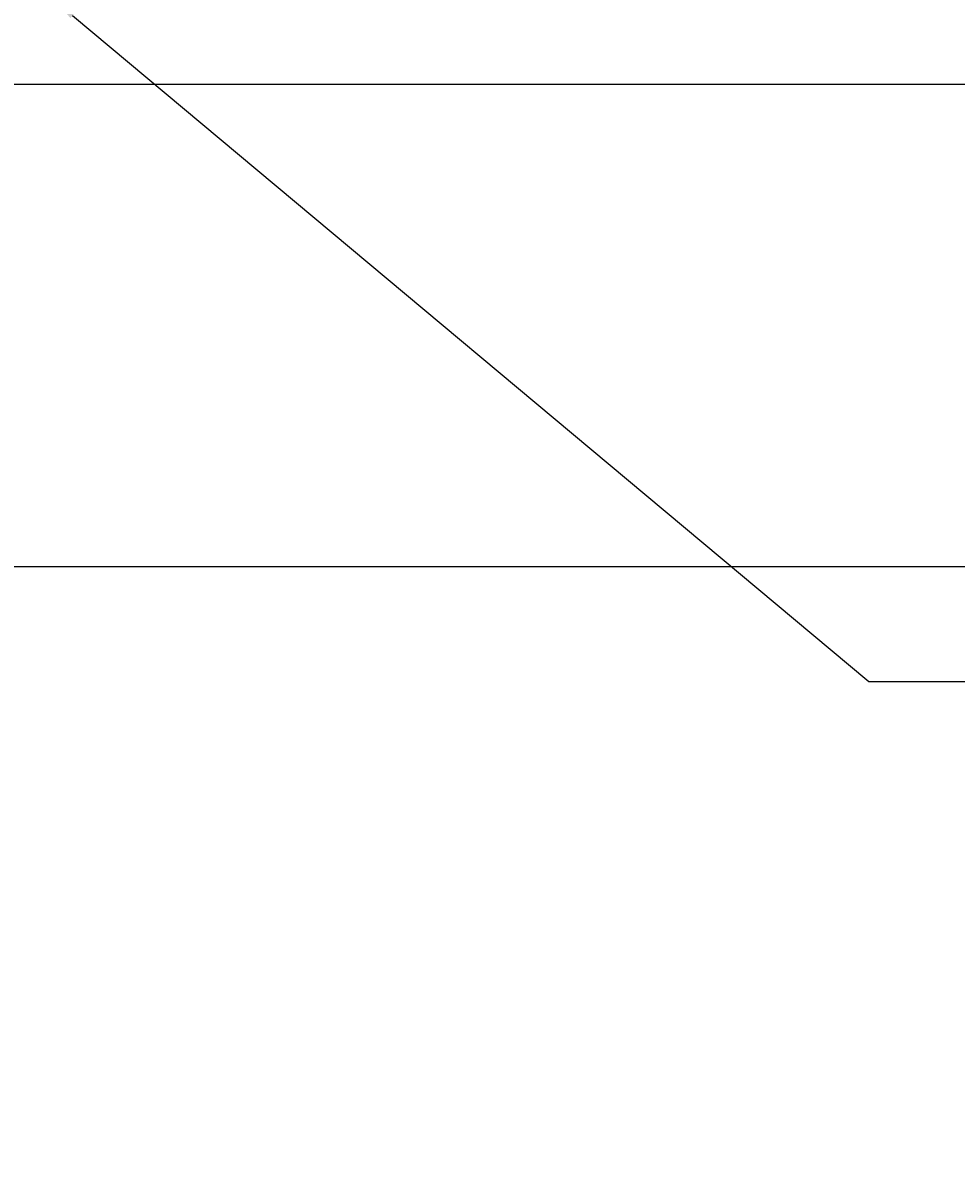
# Model space of a CAD drawing. Units: inches. Extents: x -12 to 334, y -10 to 186.
# Tile 9 of 77: x 42 to 74, y -6 to 33. Entities that reach past the tile are written whole.
import ezdxf
from ezdxf import colors
from ezdxf.entities.mleader import LeaderData, LeaderLine
from ezdxf.math import Vec2, Vec3

# ---------------------------------------------------------------- set-up
doc = ezdxf.new("R2010")
doc.units = ezdxf.units.IN
doc.header["$MEASUREMENT"] = 0
doc.layers.add('M-ANNO-TEXT', color=3, linetype='Continuous', lineweight=25)
doc.layers.add('M-DIMS', color=2, linetype='Continuous', lineweight=18)
doc.styles.get("Standard").update_dxf_attribs({"font": 'arial.ttf'})
doc.dimstyles.get("Standard").update_dxf_attribs({"dimtxt": 0.18, "dimasz": 0.18, "dimexe": 0.18, "dimexo": 0.0625, "dimgap": 0.09, "dimtad": 0, "dimtih": 1, "dimtoh": 1, "dimdec": 4, "dimzin": 0, "dimdsep": 46, "dimtxsty": 'Standard', "dimcen": 0.09, "dimadec": 0, "dimazin": 0, "dimtfac": 1, "dimtdec": 4, "dimtofl": 0, "dimtmove": 0, "dimatfit": 3, "dimfxl": 1, "dimtolj": 1, "dimtzin": 0, "dimarcsym": 0})

# ---------------------------------------------------------------- blocks, each defined once
blk = doc.blocks.new('*D1')
at = {"layer": 'Defpoints', "color": 0, "transparency": 16777216}
for p in [(281.426, 91.899), (3.376, 80.692), (281.426, 14.304)]:
    blk.add_point(p, dxfattribs=at)
at = {"layer": 'M-DIMS', "color": 0, "lineweight": -2, "transparency": 16777216}
for p, q in [((281.426, 91.836), (281.426, 14.124)), ((3.376, 80.629), (3.376, 14.124)), ((3.556, 14.304), (141.935, 14.304)), ((281.246, 14.304), (142.867, 14.304))]:
    blk.add_line(p, q, dxfattribs=at)
at = {"layer": 'M-DIMS', "color": 0, "transparency": 16777216}
for points in [[(3.556, 14.334), (3.556, 14.274), (3.376, 14.304)], [(281.246, 14.334), (281.246, 14.274), (281.426, 14.304)]]:
    blk.add_solid(points, dxfattribs=at)
at = {"layer": 'M-DIMS', "color": 0, "transparency": 16777216, "insert": (142.401, 14.304), "char_height": 0.18, "attachment_point": 5}
blk.add_mtext('\\A1;278.05', dxfattribs=at)
blk = doc.blocks.new('*D29')
at = {"layer": 'Defpoints', "color": 0, "transparency": 16777216}
for p in [(-11.174, 45.854), (221.576, 45.854), (216.576, 30.854)]:
    blk.add_point(p, dxfattribs=at)
at = {"layer": 'M-DIMS', "color": 0, "lineweight": -2, "transparency": 16777216}
for p, q in [((221.514, 45.854), (-11.354, 45.854)), ((-11.174, 45.674), (-11.174, 38.536)), ((-11.174, 31.034), (-11.174, 38.172)), ((216.514, 30.854), (-11.354, 30.854))]:
    blk.add_line(p, q, dxfattribs=at)
at = {"layer": 'M-DIMS', "color": 0, "transparency": 16777216}
for points in [[(-11.204, 45.674), (-11.144, 45.674), (-11.174, 45.854)], [(-11.204, 31.034), (-11.144, 31.034), (-11.174, 30.854)]]:
    blk.add_solid(points, dxfattribs=at)
at = {"layer": 'M-DIMS', "color": 0, "transparency": 16777216, "insert": (-11.174, 38.354), "char_height": 0.18, "attachment_point": 5}
blk.add_mtext('\\A1;15', dxfattribs=at)

msp = doc.modelspace()

# ---------------------------------------------------------------- dimensions: what is measured, and where the dimension line sits
at = {"layer": 'M-DIMS'}
dim = msp.add_linear_dim(base=(281.4256, 14.3041), p1=(3.3765, 80.6915), p2=(281.4256, 91.8988), dimstyle='Standard', override={"dimdec": 2, "dimlfac": 1, "dimrnd": 0, "dimzin": 0, "dimdsep": 46, "dimlunit": 2}, dxfattribs=at)
dim.commit()
dim.dimension.update_dxf_attribs({"geometry": '*D1', "text_midpoint": (142.401, 14.3041)})
dim = msp.add_linear_dim(base=(-11.1736, 45.8541), p1=(216.5761, 30.8541), p2=(221.5761, 45.8541), angle=90, dimstyle='Standard', override={"dimdec": 0, "dimlfac": 1, "dimrnd": 0, "dimzin": 0, "dimdsep": 46, "dimlunit": 2}, dxfattribs=at)
dim.commit()
dim.dimension.update_dxf_attribs({"geometry": '*D29', "text_midpoint": (-11.1735, 38.3541)})

# ---------------------------------------------------------------- leaders
at = {"layer": 'M-ANNO-TEXT'}
ml = msp.add_multileader_mtext('Standard', dxfattribs=at)
ml.set_content('^ICondensate outlet', color=256)
ml.set_leader_properties()
ml.build(insert=Vec2(0, 0))
ml.multileader.update_dxf_attribs({"dogleg_length": 0.36, "arrow_head_size": 0.7})
ctx = ml.context
ctx.base_point, ctx.arrow_head_size, ctx.landing_gap_size, ctx.plane_origin = Vec3(83.8784, 10.3512), 0.7, 0.09, Vec3(49.4251, 25.7584)
notes = []
notes.append((ctx, [(0, (1, 1, 0), (70.8242, 10.3512), (1, 0), 13.0542, [(0, [(42.9275, 33.6752)], 0, [])])]))
ctx.mtext.insert, ctx.mtext.flow_direction = Vec3(83.9684, 12.3853), 5
for ctx, leaders in notes:
    for number, flags, end, landing, length, lines in leaders:
        leader = LeaderData()
        leader.index, (leader.has_last_leader_line, leader.has_dogleg_vector, leader.attachment_direction) = number, flags
        leader.last_leader_point, leader.dogleg_vector, leader.dogleg_length = Vec3(end), Vec3(landing), length
        for number, points, colour, breaks in lines:
            line = LeaderLine()
            line.index, line.vertices, line.color, line.breaks = number, Vec3.list(points), colors.encode_raw_color(colour), breaks
            leader.lines.append(line)
        ctx.leaders.append(leader)

doc.saveas('drawing.dxf')
